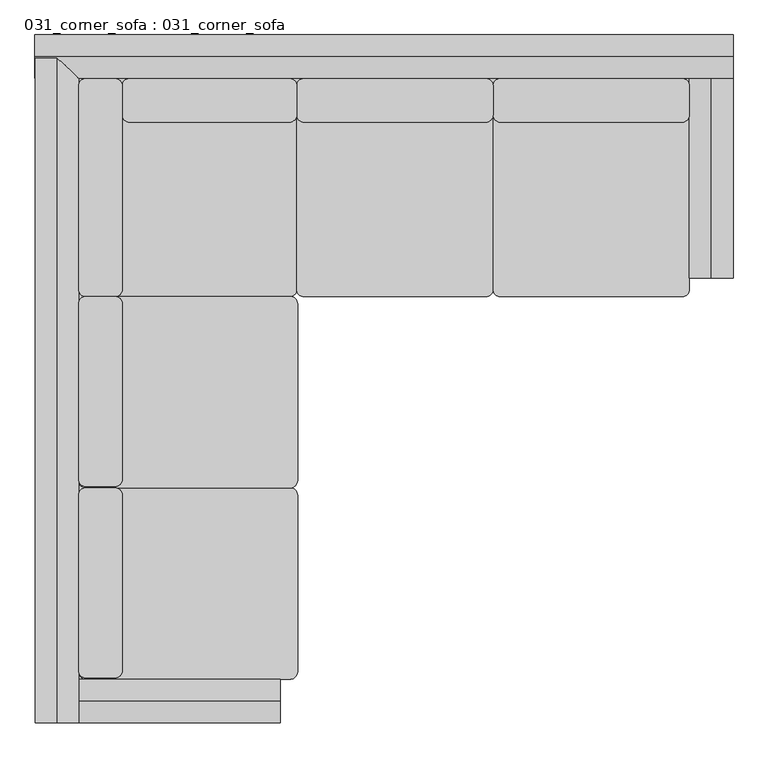
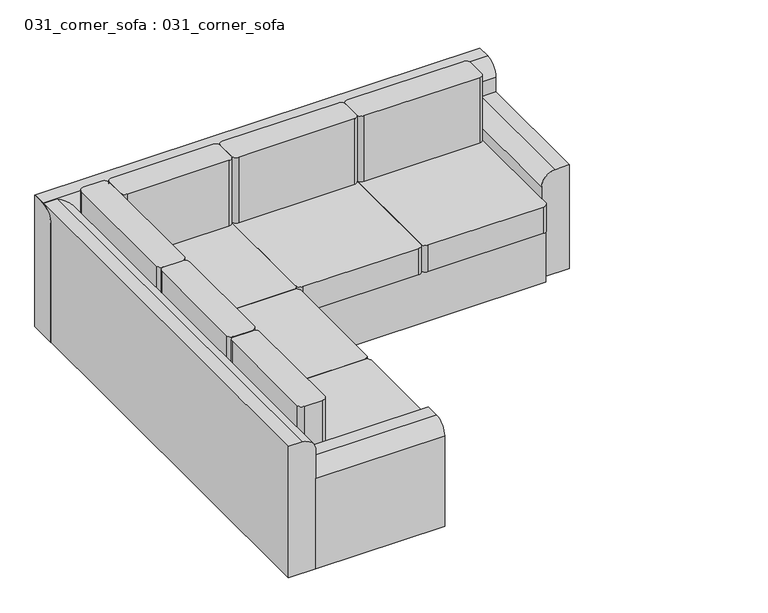
"""IFC4 building model written with IfcOpenShell, lengths in millimetres: furniture geometry, 031_corner_sofa : 031_corner_sofa."""

from ifc_helpers import new_model, si_unit, point, frame, frame_2d, origin, origin_with_axes, place, context, project, spatial, polyline, circle_curve, trimmed, segment, composite_curve, outline, extrude, source, transform, mapped, element, save


def furniture_031_corner_sofa_031_corner_sofa_f2e0ed7f(model_context):
    return source(origin(), model_context, "Body", "SweptSolid", [
        extrude(outline(polyline([(1066.8, 22.4564568), (-1066.8, 22.4564568), (-1066.8, 762.0), (1066.8, 762.0), (1066.8, 22.4564568)])), origin_with_axes(), (0.0, 0.0, 1.0), 304.8),
        extrude(outline(composite_curve([segment(polyline([(600.0, 1219.2), (600.0, 1143.0)]), True, "CONTINUOUS"), segment(trimmed(circle_curve(frame_2d((523.8, 1143.0)), 76.2), [point((600.0, 1143.0))], [point((523.8, 1066.8))], False, "CARTESIAN"), True, "CONTINUOUS"), segment(polyline([(523.8, 1066.8), (0.0, 1066.8), (0.0, 1219.2), (600.0, 1219.2)]), True, "CONTINUOUS")], self_intersect=False)), frame((0.0, 64.4, 0.0), z_axis=(0.0, 1.0, 0.0), x_axis=(0.0, 0.0, 1.0)), (0.0, 0.0, 1.0), 697.6),
        extrude(outline(polyline([(-324.8795918, 22.4564568), (-324.8795918, -1337.152522), (-1199.8102816, -1337.152522), (-1199.8102816, 22.4564568), (-324.8795918, 22.4564568)])), origin_with_axes(), (0.0, 0.0, 1.0), 304.8),
        extrude(outline(composite_curve([segment(polyline([(-1041.4, 0.0), (-327.3287994, 0.0)]), True, "CONTINUOUS"), segment(trimmed(circle_curve(frame_2d((-327.3287994, -25.4)), 25.4), [point((-327.3287994, 0.0))], [point((-301.9287994, -25.4))], False, "CARTESIAN"), True, "CONTINUOUS"), segment(polyline([(-301.9287994, -25.4), (-301.9287994, -643.176261)]), True, "CONTINUOUS"), segment(trimmed(circle_curve(frame_2d((-327.3287994, -643.176261)), 25.4), [point((-301.9287994, -643.176261))], [point((-327.3287994, -668.576261))], False, "CARTESIAN"), True, "CONTINUOUS"), segment(polyline([(-327.3287994, -668.576261), (-1041.4, -668.576261)]), True, "CONTINUOUS"), segment(trimmed(circle_curve(frame_2d((-1041.4, -643.176261)), 25.4), [point((-1041.4, -668.576261))], [point((-1066.8, -643.176261))], False, "CARTESIAN"), True, "CONTINUOUS"), segment(polyline([(-1066.8, -643.176261), (-1066.8, -25.4)]), True, "CONTINUOUS"), segment(trimmed(circle_curve(frame_2d((-1041.4, -25.4)), 25.4), [point((-1066.8, -25.4))], [point((-1041.4, 0.0))], False, "CARTESIAN"), True, "CONTINUOUS")], self_intersect=False)), frame((0.0, 0.0, 304.8), z_axis=(0.0, 0.0, 1.0), x_axis=(1.0, 0.0, 0.0)), (0.0, 0.0, 1.0), 152.4),
        extrude(outline(composite_curve([segment(polyline([(1041.4, 0.0), (406.4, 0.0)]), True, "CONTINUOUS"), segment(trimmed(circle_curve(frame_2d((406.4, 25.4)), 25.4), [point((406.4, 0.0))], [point((381.0, 25.4))], False, "CARTESIAN"), True, "CONTINUOUS"), segment(polyline([(381.0, 25.4), (381.0, 736.6)]), True, "CONTINUOUS"), segment(trimmed(circle_curve(frame_2d((406.4, 736.6)), 25.4), [point((381.0, 736.6))], [point((406.4, 762.0))], False, "CARTESIAN"), True, "CONTINUOUS"), segment(polyline([(406.4, 762.0), (1041.4, 762.0)]), True, "CONTINUOUS"), segment(trimmed(circle_curve(frame_2d((1041.4, 736.6)), 25.4), [point((1041.4, 762.0))], [point((1066.8, 736.6))], False, "CARTESIAN"), True, "CONTINUOUS"), segment(polyline([(1066.8, 736.6), (1066.8, 25.4)]), True, "CONTINUOUS"), segment(trimmed(circle_curve(frame_2d((1041.4, 25.4)), 25.4), [point((1066.8, 25.4))], [point((1041.4, 0.0))], False, "CARTESIAN"), True, "CONTINUOUS")], self_intersect=False)), frame((0.0, 0.0, 304.8), z_axis=(0.0, 0.0, 1.0), x_axis=(1.0, 0.0, 0.0)), (0.0, 0.0, 1.0), 152.4),
        extrude(outline(composite_curve([segment(polyline([(355.6, 0.0), (-279.4, 0.0)]), True, "CONTINUOUS"), segment(trimmed(circle_curve(frame_2d((-279.4, 25.4)), 25.4), [point((-279.4, 0.0))], [point((-304.8, 25.4))], False, "CARTESIAN"), True, "CONTINUOUS"), segment(polyline([(-304.8, 25.4), (-304.8, 736.6)]), True, "CONTINUOUS"), segment(trimmed(circle_curve(frame_2d((-279.4, 736.6)), 25.4), [point((-304.8, 736.6))], [point((-279.4, 762.0))], False, "CARTESIAN"), True, "CONTINUOUS"), segment(polyline([(-279.4, 762.0), (355.6, 762.0)]), True, "CONTINUOUS"), segment(trimmed(circle_curve(frame_2d((355.6, 736.6)), 25.4), [point((355.6, 762.0))], [point((381.0, 736.6))], False, "CARTESIAN"), True, "CONTINUOUS"), segment(polyline([(381.0, 736.6), (381.0, 25.4)]), True, "CONTINUOUS"), segment(trimmed(circle_curve(frame_2d((355.6, 25.4)), 25.4), [point((381.0, 25.4))], [point((355.6, 0.0))], False, "CARTESIAN"), True, "CONTINUOUS")], self_intersect=False)), frame((0.0, 0.0, 304.8), z_axis=(0.0, 0.0, 1.0), x_axis=(1.0, 0.0, 0.0)), (0.0, 0.0, 1.0), 152.4),
        extrude(outline(composite_curve([segment(polyline([(-330.2, 0.0), (-1041.4, 0.0)]), True, "CONTINUOUS"), segment(trimmed(circle_curve(frame_2d((-1041.4, 25.4)), 25.4), [point((-1041.4, 0.0))], [point((-1066.8, 25.4))], False, "CARTESIAN"), True, "CONTINUOUS"), segment(polyline([(-1066.8, 25.4), (-1066.8, 736.6)]), True, "CONTINUOUS"), segment(trimmed(circle_curve(frame_2d((-1041.4, 736.6)), 25.4), [point((-1066.8, 736.6))], [point((-1041.4, 762.0))], False, "CARTESIAN"), True, "CONTINUOUS"), segment(polyline([(-1041.4, 762.0), (-330.2, 762.0)]), True, "CONTINUOUS"), segment(trimmed(circle_curve(frame_2d((-330.2, 736.6)), 25.4), [point((-330.2, 762.0))], [point((-304.8, 736.6))], False, "CARTESIAN"), True, "CONTINUOUS"), segment(polyline([(-304.8, 736.6), (-304.8, 25.4)]), True, "CONTINUOUS"), segment(trimmed(circle_curve(frame_2d((-330.2, 25.4)), 25.4), [point((-304.8, 25.4))], [point((-330.2, 0.0))], False, "CARTESIAN"), True, "CONTINUOUS")], self_intersect=False)), frame((0.0, 0.0, 304.8), z_axis=(0.0, 0.0, 1.0), x_axis=(1.0, 0.0, 0.0)), (0.0, 0.0, 1.0), 152.4),
        extrude(outline(composite_curve([segment(polyline([(-939.8, -664.3639266), (-1041.4, -664.3639266)]), True, "CONTINUOUS"), segment(trimmed(circle_curve(frame_2d((-1041.4, -638.9639266)), 25.4), [point((-1041.4, -664.3639266))], [point((-1066.8, -638.9639266))], False, "CARTESIAN"), True, "CONTINUOUS"), segment(polyline([(-1066.8, -638.9639266), (-1066.8, -25.4)]), True, "CONTINUOUS"), segment(trimmed(circle_curve(frame_2d((-1041.4, -25.4)), 25.4), [point((-1066.8, -25.4))], [point((-1041.4, 0.0))], False, "CARTESIAN"), True, "CONTINUOUS"), segment(polyline([(-1041.4, 0.0), (-939.8, 0.0)]), True, "CONTINUOUS"), segment(trimmed(circle_curve(frame_2d((-939.8, -25.4)), 25.4), [point((-939.8, 0.0))], [point((-914.4, -25.4))], False, "CARTESIAN"), True, "CONTINUOUS"), segment(polyline([(-914.4, -25.4), (-914.4, -638.9639266)]), True, "CONTINUOUS"), segment(trimmed(circle_curve(frame_2d((-939.8, -638.9639266)), 25.4), [point((-914.4, -638.9639266))], [point((-939.8, -664.3639266))], False, "CARTESIAN"), True, "CONTINUOUS")], self_intersect=False)), frame((0.0, 0.0, 457.2), z_axis=(0.0, 0.0, 1.0), x_axis=(1.0, 0.0, 0.0)), (0.0, 0.0, 1.0), 381.0),
        extrude(outline(composite_curve([segment(polyline([(-939.8, 0.0), (-1041.4, 0.0)]), True, "CONTINUOUS"), segment(trimmed(circle_curve(frame_2d((-1041.4, 25.4)), 25.4), [point((-1041.4, 0.0))], [point((-1066.8, 25.4))], False, "CARTESIAN"), True, "CONTINUOUS"), segment(polyline([(-1066.8, 25.4), (-1066.8, 736.6)]), True, "CONTINUOUS"), segment(trimmed(circle_curve(frame_2d((-1041.4, 736.6)), 25.4), [point((-1066.8, 736.6))], [point((-1041.4, 762.0))], False, "CARTESIAN"), True, "CONTINUOUS"), segment(polyline([(-1041.4, 762.0), (-939.8, 762.0)]), True, "CONTINUOUS"), segment(trimmed(circle_curve(frame_2d((-939.8, 736.6)), 25.4), [point((-939.8, 762.0))], [point((-914.4, 736.6))], False, "CARTESIAN"), True, "CONTINUOUS"), segment(polyline([(-914.4, 736.6), (-914.4, 25.4)]), True, "CONTINUOUS"), segment(trimmed(circle_curve(frame_2d((-939.8, 25.4)), 25.4), [point((-914.4, 25.4))], [point((-939.8, 0.0))], False, "CARTESIAN"), True, "CONTINUOUS")], self_intersect=False)), frame((0.0, 0.0, 457.2), z_axis=(0.0, 0.0, 1.0), x_axis=(1.0, 0.0, 0.0)), (0.0, 0.0, 1.0), 381.0),
        extrude(outline(composite_curve([segment(polyline([(-330.2, 609.6), (-889.0, 609.6)]), True, "CONTINUOUS"), segment(trimmed(circle_curve(frame_2d((-889.0, 635.0)), 25.4), [point((-889.0, 609.6))], [point((-914.4, 635.0))], False, "CARTESIAN"), True, "CONTINUOUS"), segment(polyline([(-914.4, 635.0), (-914.4, 736.6)]), True, "CONTINUOUS"), segment(trimmed(circle_curve(frame_2d((-889.0, 736.6)), 25.4), [point((-914.4, 736.6))], [point((-889.0, 762.0))], False, "CARTESIAN"), True, "CONTINUOUS"), segment(polyline([(-889.0, 762.0), (-330.2, 762.0)]), True, "CONTINUOUS"), segment(trimmed(circle_curve(frame_2d((-330.2, 736.6)), 25.4), [point((-330.2, 762.0))], [point((-304.8, 736.6))], False, "CARTESIAN"), True, "CONTINUOUS"), segment(polyline([(-304.8, 736.6), (-304.8, 635.0)]), True, "CONTINUOUS"), segment(trimmed(circle_curve(frame_2d((-330.2, 635.0)), 25.4), [point((-304.8, 635.0))], [point((-330.2, 609.6))], False, "CARTESIAN"), True, "CONTINUOUS")], self_intersect=False)), frame((0.0, 0.0, 457.2), z_axis=(0.0, 0.0, 1.0), x_axis=(1.0, 0.0, 0.0)), (0.0, 0.0, 1.0), 381.0),
        extrude(outline(composite_curve([segment(trimmed(circle_curve(frame_2d((355.6, 736.6)), 25.4), [point((355.6, 762.0))], [point((381.0, 736.6))], False, "CARTESIAN"), True, "CONTINUOUS"), segment(polyline([(381.0, 736.6), (381.0, 635.0)]), True, "CONTINUOUS"), segment(trimmed(circle_curve(frame_2d((355.6, 635.0)), 25.4), [point((381.0, 635.0))], [point((355.6, 609.6))], False, "CARTESIAN"), True, "CONTINUOUS"), segment(polyline([(355.6, 609.6), (-279.4, 609.6)]), True, "CONTINUOUS"), segment(trimmed(circle_curve(frame_2d((-279.4, 635.0)), 25.4), [point((-279.4, 609.6))], [point((-304.8, 635.0))], False, "CARTESIAN"), True, "CONTINUOUS"), segment(polyline([(-304.8, 635.0), (-304.8, 736.6)]), True, "CONTINUOUS"), segment(trimmed(circle_curve(frame_2d((-279.4, 736.6)), 25.4), [point((-304.8, 736.6))], [point((-279.4, 762.0))], False, "CARTESIAN"), True, "CONTINUOUS"), segment(polyline([(-279.4, 762.0), (355.6, 762.0)]), True, "CONTINUOUS")], self_intersect=False)), frame((0.0, 0.0, 457.2), z_axis=(0.0, 0.0, 1.0), x_axis=(1.0, 0.0, 0.0)), (0.0, 0.0, 1.0), 381.0),
        extrude(outline(composite_curve([segment(trimmed(circle_curve(frame_2d((1041.4, 736.6)), 25.4), [point((1041.4, 762.0))], [point((1066.8, 736.6))], False, "CARTESIAN"), True, "CONTINUOUS"), segment(polyline([(1066.8, 736.6), (1066.8, 635.0)]), True, "CONTINUOUS"), segment(trimmed(circle_curve(frame_2d((1041.4, 635.0)), 25.4), [point((1066.8, 635.0))], [point((1041.4, 609.6))], False, "CARTESIAN"), True, "CONTINUOUS"), segment(polyline([(1041.4, 609.6), (406.4, 609.6)]), True, "CONTINUOUS"), segment(trimmed(circle_curve(frame_2d((406.4, 635.0)), 25.4), [point((406.4, 609.6))], [point((381.0, 635.0))], False, "CARTESIAN"), True, "CONTINUOUS"), segment(polyline([(381.0, 635.0), (381.0, 736.6)]), True, "CONTINUOUS"), segment(trimmed(circle_curve(frame_2d((406.4, 736.6)), 25.4), [point((381.0, 736.6))], [point((406.4, 762.0))], False, "CARTESIAN"), True, "CONTINUOUS"), segment(polyline([(406.4, 762.0), (1041.4, 762.0)]), True, "CONTINUOUS")], self_intersect=False)), frame((0.0, 0.0, 457.2), z_axis=(0.0, 0.0, 1.0), x_axis=(1.0, 0.0, 0.0)), (0.0, 0.0, 1.0), 381.0),
        extrude(outline(composite_curve([segment(polyline([(-1041.4, -668.576261), (-327.3287994, -668.576261)]), True, "CONTINUOUS"), segment(trimmed(circle_curve(frame_2d((-327.3287994, -693.976261)), 25.4), [point((-327.3287994, -668.576261))], [point((-301.9287994, -693.976261))], False, "CARTESIAN"), True, "CONTINUOUS"), segment(polyline([(-301.9287994, -693.976261), (-301.9287994, -1311.752522)]), True, "CONTINUOUS"), segment(trimmed(circle_curve(frame_2d((-327.3287994, -1311.752522)), 25.4), [point((-301.9287994, -1311.752522))], [point((-327.3287994, -1337.152522))], False, "CARTESIAN"), True, "CONTINUOUS"), segment(polyline([(-327.3287994, -1337.152522), (-1041.4, -1337.152522)]), True, "CONTINUOUS"), segment(trimmed(circle_curve(frame_2d((-1041.4, -1311.752522)), 25.4), [point((-1041.4, -1337.152522))], [point((-1066.8, -1311.752522))], False, "CARTESIAN"), True, "CONTINUOUS"), segment(polyline([(-1066.8, -1311.752522), (-1066.8, -693.976261)]), True, "CONTINUOUS"), segment(trimmed(circle_curve(frame_2d((-1041.4, -693.976261)), 25.4), [point((-1066.8, -693.976261))], [point((-1041.4, -668.576261))], False, "CARTESIAN"), True, "CONTINUOUS")], self_intersect=False)), frame((0.0, 0.0, 304.8), z_axis=(0.0, 0.0, 1.0), x_axis=(1.0, 0.0, 0.0)), (0.0, 0.0, 1.0), 152.4),
        extrude(outline(composite_curve([segment(polyline([(-939.8, -1332.9401876), (-1041.4, -1332.9401876)]), True, "CONTINUOUS"), segment(trimmed(circle_curve(frame_2d((-1041.4, -1307.5401876)), 25.4), [point((-1041.4, -1332.9401876))], [point((-1066.8, -1307.5401876))], False, "CARTESIAN"), True, "CONTINUOUS"), segment(polyline([(-1066.8, -1307.5401876), (-1066.8, -693.976261)]), True, "CONTINUOUS"), segment(trimmed(circle_curve(frame_2d((-1041.4, -693.976261)), 25.4), [point((-1066.8, -693.976261))], [point((-1041.4, -668.576261))], False, "CARTESIAN"), True, "CONTINUOUS"), segment(polyline([(-1041.4, -668.576261), (-939.8, -668.576261)]), True, "CONTINUOUS"), segment(trimmed(circle_curve(frame_2d((-939.8, -693.976261)), 25.4), [point((-939.8, -668.576261))], [point((-914.4, -693.976261))], False, "CARTESIAN"), True, "CONTINUOUS"), segment(polyline([(-914.4, -693.976261), (-914.4, -1307.5401876)]), True, "CONTINUOUS"), segment(trimmed(circle_curve(frame_2d((-939.8, -1307.5401876)), 25.4), [point((-914.4, -1307.5401876))], [point((-939.8, -1332.9401876))], False, "CARTESIAN"), True, "CONTINUOUS")], self_intersect=False)), frame((0.0, 0.0, 457.2), z_axis=(0.0, 0.0, 1.0), x_axis=(1.0, 0.0, 0.0)), (0.0, 0.0, 1.0), 381.0),
        extrude(outline(composite_curve([segment(polyline([(-1337.152522, 600.0), (-1337.152522, 0.0), (-1489.552522, 0.0), (-1489.552522, 523.8)]), True, "CONTINUOUS"), segment(trimmed(circle_curve(frame_2d((-1413.352522, 523.8)), 76.2), [point((-1489.552522, 523.8))], [point((-1413.352522, 600.0))], False, "CARTESIAN"), True, "CONTINUOUS"), segment(polyline([(-1413.352522, 600.0), (-1337.152522, 600.0)]), True, "CONTINUOUS")], self_intersect=False)), frame((-1066.8, 0.0, 0.0), z_axis=(1.0, 0.0, 0.0), x_axis=(0.0, 1.0, 0.0)), (0.0, 0.0, 1.0), 704.4455993),
        extrude(outline(composite_curve([segment(polyline([(762.8736306, 0.0), (762.8736306, 685.8)]), True, "CONTINUOUS"), segment(trimmed(circle_curve(frame_2d((839.0736306, 685.8)), 76.2), [point((762.8736306, 685.8))], [point((839.0736306, 762.0))], False, "CARTESIAN"), True, "CONTINUOUS"), segment(polyline([(839.0736306, 762.0), (914.4, 762.0), (914.4, 0.0), (762.8736306, 0.0)]), True, "CONTINUOUS")], self_intersect=False)), frame((-1219.2, 0.0, 0.0), z_axis=(1.0, 0.0, 0.0), x_axis=(0.0, 1.0, 0.0)), (0.0, 0.0, 1.0), 2438.4),
        extrude(outline(composite_curve([segment(polyline([(0.0, -1066.8), (685.8, -1066.8)]), True, "CONTINUOUS"), segment(trimmed(circle_curve(frame_2d((685.8, -1143.0)), 76.2), [point((685.8, -1066.8))], [point((762.0, -1143.0))], False, "CARTESIAN"), True, "CONTINUOUS"), segment(polyline([(762.0, -1143.0), (762.0, -1218.3263694), (0.0, -1218.3263694), (0.0, -1066.8)]), True, "CONTINUOUS")], self_intersect=False)), frame((0.0, -1489.552522, 0.0), z_axis=(0.0, 1.0, 0.0), x_axis=(0.0, 0.0, 1.0)), (0.0, 0.0, 1.0), 2403.952522),
    ])


if __name__ == "__main__":
    model = new_model("IFC4")
    model_context = context("Model", 3, world=origin())
    ifc_project = project(units=[si_unit("LENGTHUNIT", "METRE", prefix="MILLI")], contexts=[model_context])
    site = spatial("IfcSite", under=ifc_project)
    building = spatial("IfcBuilding", under=site)
    placement = place(None, origin())
    furniture_031_corner_sofa_031_corner_sofa_shape = furniture_031_corner_sofa_031_corner_sofa_f2e0ed7f(model_context)
    element("IfcFurniture", 1, ObjectType="031_corner_sofa : 031_corner_sofa", at=placement, inside=building, context=model_context, shape_type="MappedRepresentation", body=[
        mapped(furniture_031_corner_sofa_031_corner_sofa_shape, transform((0.0, 0.0, 0.0), x_axis=(1.0, 0.0, 0.0), y_axis=(0.0, 1.0, 0.0), z_axis=(0.0, 0.0, 1.0))),
    ])
    save(model, "model.ifc")

# Revit data of these elements
# Type "031_corner_sofa : 031_corner_sofa"
#   Default Elevation = 0
